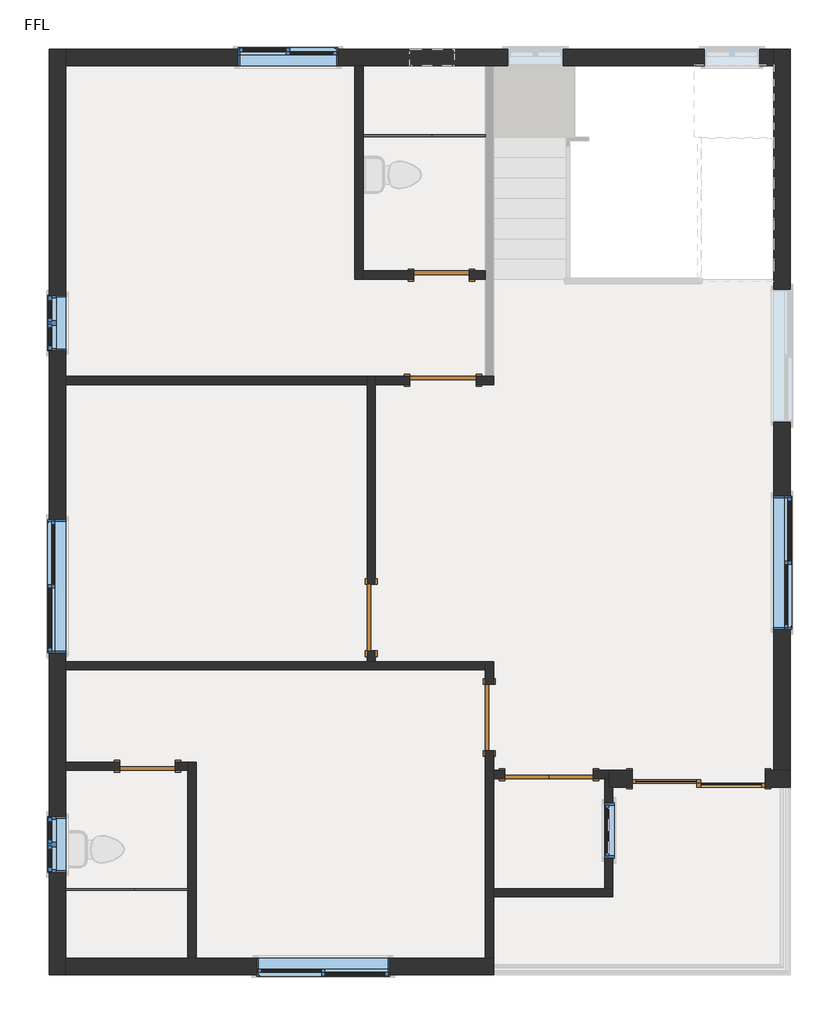
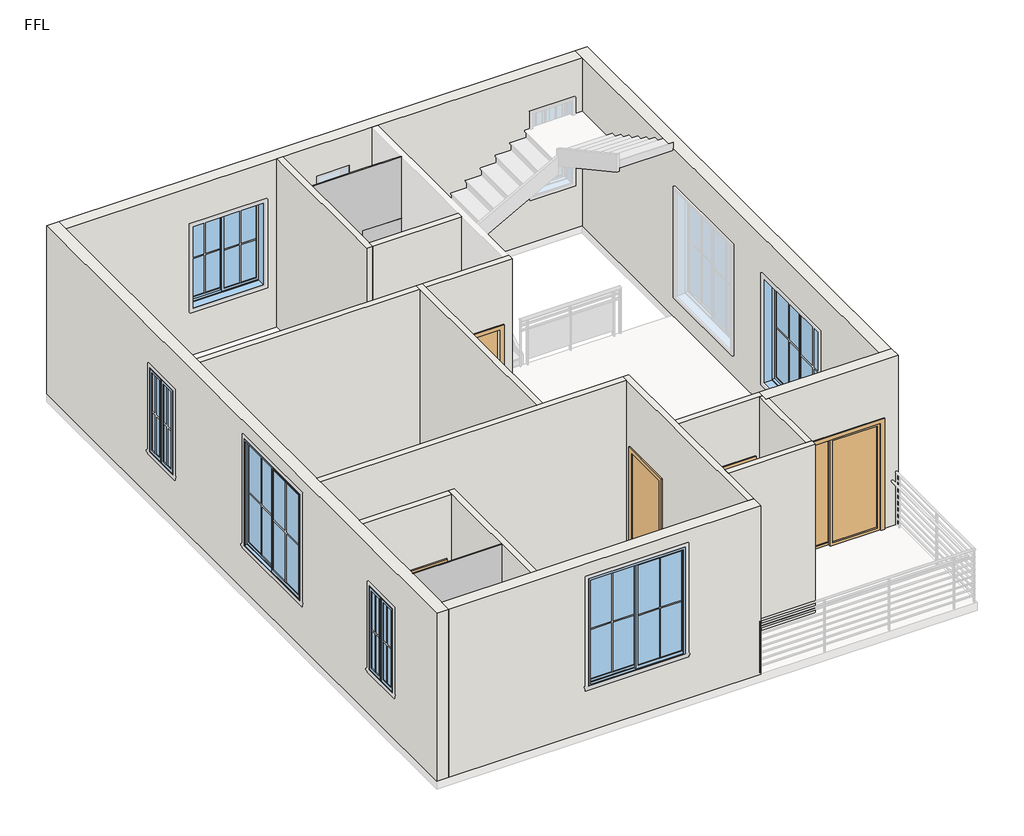
# One storey, part 1 of 3: 17 walls, 7 doors, 7 windows, 4 plates.
"""IFC4 building model written with IfcOpenShell, lengths in millimetres."""

from ifc_helpers import new_model, si_unit, frame, origin, place, context, project, spatial, polyline, outline, extrude, faceted_brep, transform, mapped, element, save
from components import door_eb8a45e1, door_d4d75d1e, door_d8f5dbb5, door_f2b275c1, door_5e62189b, door_17d80c48, system_panel_glazed_b407a8af, system_panel_glazed_ca5a80b0, window_9dcce3b5, window_5a369d27, window_5810691a, window_sliding_double_6_x7_726fea71

model = new_model("IFC4")

# Units and contexts
model_context = context("Model", 3, world=origin())
ifc_project = project(units=[si_unit("LENGTHUNIT", "METRE", prefix="MILLI")], contexts=[model_context])

# Site, building, storey
site = spatial("IfcSite", under=ifc_project)
building = spatial("IfcBuilding", under=site)
storey = spatial("IfcBuildingStorey", under=building, Name="FFL", Elevation=3505.2)

# Doors
placement = place(None, origin())
door_shape = door_eb8a45e1(model_context)
element("IfcDoor", 1, ObjectType="Door-Double-Flush_Panel : 48\" x 84\"", at=placement, inside=storey, context=model_context, shape_type="MappedRepresentation", body=[
    mapped(door_shape, transform((-7052.0133719, 2428.2295268, 3505.2), x_axis=(-1.0, 0.0, 0.0), y_axis=(0.0, -1.0, 0.0), z_axis=(0.0, 0.0, 1.0))),
])
door_2_shape = door_d4d75d1e(model_context)
element("IfcDoor", 2, ObjectType="Door-Double-Sliding : 72\" x 84\"", at=placement, inside=storey, context=model_context, shape_type="MappedRepresentation", body=[
    mapped(door_2_shape, transform((-4993.0257748, 2498.0795268, 3505.2), x_axis=(-1.0, 0.0, 0.0), y_axis=(0.0, -1.0, 0.0), z_axis=(0.0, 0.0, 1.0))),
])
door_3_shape = door_d8f5dbb5(model_context)
element("IfcDoor", 3, ObjectType="Single-Flush : 30\" x 80\"", at=placement, inside=storey, context=model_context, shape_type="MappedRepresentation", body=[
    mapped(door_3_shape, transform((-8533.1502526, 9296.8628699, 3505.2), x_axis=(1.0, 0.0, 0.0), y_axis=(0.0, 1.0, 0.0), z_axis=(0.0, 0.0, 1.0))),
])
door_4_shape = door_f2b275c1(model_context)
element("IfcDoor", 4, ObjectType="Single-Flush : 30\" x 80\"", at=placement, inside=storey, context=model_context, shape_type="MappedRepresentation", body=[
    mapped(door_4_shape, transform((-12571.8381491, 2542.5295268, 3505.2), x_axis=(1.0, 0.0, 0.0), y_axis=(0.0, 1.0, 0.0), z_axis=(0.0, 0.0, 1.0))),
])
door_5_shape = door_5e62189b(model_context)
element("IfcDoor", 5, ObjectType="Single-Flush : 36\" x 80\"", at=placement, inside=storey, context=model_context, shape_type="MappedRepresentation", body=[
    mapped(door_5_shape, transform((-9498.3502612, 4585.1627283, 3505.2), x_axis=(0.0, -1.0, 0.0), y_axis=(1.0, 0.0, 0.0), z_axis=(0.0, 0.0, 1.0))),
])
door_6_shape = door_17d80c48(model_context)
element("IfcDoor", 6, ObjectType="Single-Flush : 36\" x 80\"", at=placement, inside=storey, context=model_context, shape_type="MappedRepresentation", body=[
    mapped(door_6_shape, transform((-7872.750969, 3213.5627283, 3505.2), x_axis=(0.0, 1.0, 0.0), y_axis=(-1.0, 0.0, 0.0), z_axis=(0.0, 0.0, 1.0))),
])
element("IfcDoor", 7, ObjectType="Single-Flush : 36\" x 80\"", at=placement, inside=storey, context=model_context, shape_type="MappedRepresentation", body=[
    mapped(door_6_shape, transform((-8507.7502526, 7849.0628362, 3505.2), x_axis=(1.0, 0.0, 0.0), y_axis=(0.0, 1.0, 0.0), z_axis=(0.0, 0.0, 1.0))),
])

# Plates
system_panel_glazed_shape = system_panel_glazed_b407a8af(model_context)
element("IfcPlate", 8, ObjectType="System Panel : Glazed", at=placement, inside=storey, context=model_context, shape_type="MappedRepresentation", body=[
    mapped(system_panel_glazed_shape, transform((-12387.6881491, 816.3157145, 3505.2), x_axis=(1.0, 0.0, 0.0), y_axis=(0.0, 1.0, 0.0), z_axis=(0.0, 0.0, 1.0))),
])
element("IfcPlate", 9, ObjectType="System Panel : Glazed", at=placement, inside=storey, context=model_context, shape_type="MappedRepresentation", body=[
    mapped(system_panel_glazed_shape, transform((-8298.2002526, 11182.8127591, 3505.2), x_axis=(1.0, 0.0, 0.0), y_axis=(0.0, 1.0, 0.0), z_axis=(0.0, 0.0, 1.0))),
])
system_panel_glazed_2_shape = system_panel_glazed_ca5a80b0(model_context)
element("IfcPlate", 10, ObjectType="System Panel : Glazed", at=placement, inside=storey, context=model_context, shape_type="MappedRepresentation", body=[
    mapped(system_panel_glazed_2_shape, transform((-12857.5442008, 816.3157145, 3505.2), x_axis=(1.0, 0.0, 0.0), y_axis=(0.0, 1.0, 0.0), z_axis=(0.0, 0.0, 1.0))),
])
element("IfcPlate", 11, ObjectType="System Panel : Glazed", at=placement, inside=storey, context=model_context, shape_type="MappedRepresentation", body=[
    mapped(system_panel_glazed_2_shape, transform((-8768.1005763, 11182.8127591, 3505.2), x_axis=(1.0, 0.0, 0.0), y_axis=(0.0, 1.0, 0.0), z_axis=(0.0, 0.0, 1.0))),
])

# Walls
element("IfcWall", 12, ObjectType="10\"", at=placement, inside=storey, context=model_context, shape_type="Brep", body=[
    faceted_brep([(-13924.3002526, 12402.0128362, 3505.2), (-13924.3002526, -323.3871638, 3505.2), (-13924.3002526, -323.3871638, 6858.0), (-13924.3002526, 12402.0128362, 6858.0), (-13924.3002526, 5931.3627283, 6553.2), (-13924.3002526, 4102.5627283, 6553.2), (-13924.3002526, 4102.5627283, 4419.6), (-13924.3002526, 5931.3627283, 4419.6), (-13924.3002526, 9017.4628362, 6096.0), (-13924.3002526, 8255.4628362, 6096.0), (-13924.3002526, 8255.4628362, 4419.6), (-13924.3002526, 9017.4628362, 4419.6), (-13924.3002526, 1848.3128362, 6096.0), (-13924.3002526, 1086.3128362, 6096.0), (-13924.3002526, 1086.3128362, 4419.6), (-13924.3002526, 1848.3128362, 4419.6), (-13695.7002526, 12402.0128362, 3505.2), (-13695.7002526, 12402.0128362, 6858.0), (-13695.7002526, 12173.4128362, 6858.0), (-13695.7002526, 7906.2128362, 6858.0), (-13695.7002526, 7791.9128362, 6858.0), (-13695.7002526, 3981.9127283, 6858.0), (-13695.7002526, 3867.6127283, 6858.0), (-13695.7002526, 2599.6795268, 6858.0), (-13695.7002526, 2485.3795268, 6858.0), (-13695.7002526, -94.7871638, 6858.0), (-13695.7002526, -323.3871638, 6858.0), (-13695.7002526, -323.3871638, 3505.2), (-13695.7002526, -94.7871638, 3505.2), (-13695.7002526, 2485.3795268, 3505.2), (-13695.7002526, 2599.6795268, 3505.2), (-13695.7002526, 3867.6127283, 3505.2), (-13695.7002526, 3981.9127283, 3505.2), (-13695.7002526, 7791.9128362, 3505.2), (-13695.7002526, 7906.2128362, 3505.2), (-13695.7002526, 12173.4128362, 3505.2), (-13695.7002526, 5931.3627283, 6553.2), (-13695.7002526, 5931.3627283, 4419.6), (-13695.7002526, 4102.5627283, 4419.6), (-13695.7002526, 4102.5627283, 6553.2), (-13695.7002526, 9017.4628362, 6096.0), (-13695.7002526, 9017.4628362, 4419.6), (-13695.7002526, 8255.4628362, 4419.6), (-13695.7002526, 8255.4628362, 6096.0), (-13695.7002526, 1848.3128362, 6096.0), (-13695.7002526, 1848.3128362, 4419.6), (-13695.7002526, 1086.3128362, 4419.6), (-13695.7002526, 1086.3128362, 6096.0)], [[[0, 1, 2, 3], [4, 5, 6, 7], [8, 9, 10, 11], [12, 13, 14, 15]], [[16, 17, 18, 19, 20, 21, 22, 23, 24, 25, 26, 27, 28, 29, 30, 31, 32, 33, 34, 35], [36, 37, 38, 39], [40, 41, 42, 43], [44, 45, 46, 47]], [[1, 0, 16, 35, 34, 33, 32, 31, 30, 29, 28, 27]], [[3, 2, 26, 25, 24, 23, 22, 21, 20, 19, 18, 17]], [[2, 1, 27, 26]], [[0, 3, 17, 16]], [[37, 36, 4, 7]], [[38, 37, 7, 6]], [[39, 38, 6, 5]], [[36, 39, 5, 4]], [[41, 40, 8, 11]], [[42, 41, 11, 10]], [[43, 42, 10, 9]], [[40, 43, 9, 8]], [[45, 44, 12, 15]], [[46, 45, 15, 14]], [[47, 46, 14, 13]], [[44, 47, 13, 12]]]),
])
element("IfcWall", 13, ObjectType="10\"", at=placement, inside=storey, context=model_context, shape_type="Brep", body=[
    faceted_brep([(-13695.7002526, -323.3871638, 3505.2), (-7815.600969, -323.3871638, 3505.2), (-7815.600969, -323.3871638, 6858.0), (-13695.7002526, -323.3871638, 6858.0), (-11073.150969, -323.3871638, 6553.2), (-9244.350969, -323.3871638, 6553.2), (-9244.350969, -323.3871638, 4419.6), (-11073.150969, -323.3871638, 4419.6), (-13695.7002526, -94.7871638, 3505.2), (-13695.7002526, -94.7871638, 6858.0), (-12019.3881491, -94.7871638, 6858.0), (-11905.0881491, -94.7871638, 6858.0), (-7929.900969, -94.7871638, 6858.0), (-7815.600969, -94.7871638, 6858.0), (-7815.600969, -94.7871638, 3505.2), (-7929.900969, -94.7871638, 3505.2), (-11905.0881491, -94.7871638, 3505.2), (-12019.3881491, -94.7871638, 3505.2), (-11073.150969, -94.7871638, 6553.2), (-11073.150969, -94.7871638, 4419.6), (-9244.350969, -94.7871638, 4419.6), (-9244.350969, -94.7871638, 6553.2)], [[[0, 1, 2, 3], [4, 5, 6, 7]], [[8, 9, 10, 11, 12, 13, 14, 15, 16, 17], [18, 19, 20, 21]], [[1, 0, 8, 17, 16, 15, 14]], [[3, 2, 13, 12, 11, 10, 9]], [[0, 3, 9, 8]], [[2, 1, 14, 13]], [[19, 18, 4, 7]], [[20, 19, 7, 6]], [[21, 20, 6, 5]], [[18, 21, 5, 4]]]),
])
element("IfcWall", 14, ObjectType="10\"", at=placement, inside=storey, context=model_context, shape_type="Brep", body=[
    faceted_brep([(-6231.2757748, 2256.7795268, 3505.2), (-6174.1257748, 2256.7795268, 3505.2), (-5907.4257748, 2256.7795268, 3505.2), (-5907.4257748, 2256.7795268, 5638.8), (-4078.6257748, 2256.7795268, 5638.8), (-4078.6257748, 2256.7795268, 3505.2), (-3735.7257748, 2256.7795268, 3505.2), (-3735.7257748, 2256.7795268, 6858.0), (-6174.1257748, 2256.7795268, 6858.0), (-6231.2757748, 2256.7795268, 6858.0), (-5907.4257748, 2485.3795268, 5638.8), (-5907.4257748, 2485.3795268, 3505.2), (-6231.2757748, 2485.3795268, 3505.2), (-6231.2757748, 2485.3795268, 6858.0), (-3964.3257748, 2485.3795268, 6858.0), (-3735.7257748, 2485.3795268, 6858.0), (-3735.7257748, 2485.3795268, 3505.2), (-3964.3257748, 2485.3795268, 3505.2), (-4078.6257748, 2485.3795268, 3505.2), (-4078.6257748, 2485.3795268, 5638.8), (-6231.2757748, 2371.0795268, 3505.2), (-6231.2757748, 2371.0795268, 6858.0)], [[[0, 1, 2, 3, 4, 5, 6, 7, 8, 9]], [[10, 11, 12, 13, 14, 15, 16, 17, 18, 19]], [[12, 11, 2, 1, 0, 20]], [[18, 17, 16, 6, 5]], [[9, 8, 7, 15, 14, 13, 21]], [[0, 9, 21, 13, 12, 20]], [[7, 6, 16, 15]], [[5, 4, 19, 18]], [[3, 2, 11, 10]], [[4, 3, 10, 19]]]),
])
element("IfcWall", 15, ObjectType="10\"", at=placement, inside=storey, context=model_context, shape_type="Brep", body=[
    faceted_brep([(-3735.7257748, 2485.3795268, 3505.2), (-3735.7257748, 12402.0128362, 3505.2), (-3735.7257748, 12402.0128362, 6858.0), (-3735.7257748, 2485.3795268, 6858.0), (-3735.7257748, 4428.4795268, 6096.0), (-3735.7257748, 6257.2795268, 6096.0), (-3735.7257748, 6257.2795268, 3962.4), (-3735.7257748, 4428.4795268, 3962.4), (-3735.7257748, 7273.2795268, 6096.0), (-3735.7257748, 9102.0795268, 6096.0), (-3735.7257748, 9102.0795268, 3962.4), (-3735.7257748, 7273.2795268, 3962.4), (-3964.3257748, 2485.3795268, 3505.2), (-3964.3257748, 2485.3795268, 6858.0), (-3964.3257748, 12173.4128362, 6858.0), (-3964.3257748, 12402.0128362, 6858.0), (-3964.3257748, 12402.0128362, 3505.2), (-3964.3257748, 12173.4128362, 3505.2), (-3964.3257748, 4428.4795268, 6096.0), (-3964.3257748, 4428.4795268, 3962.4), (-3964.3257748, 6257.2795268, 3962.4), (-3964.3257748, 6257.2795268, 6096.0), (-3964.3257748, 7273.2795268, 6096.0), (-3964.3257748, 7273.2795268, 3962.4), (-3964.3257748, 9102.0795268, 3962.4), (-3964.3257748, 9102.0795268, 6096.0)], [[[0, 1, 2, 3], [4, 5, 6, 7], [8, 9, 10, 11]], [[12, 13, 14, 15, 16, 17], [18, 19, 20, 21], [22, 23, 24, 25]], [[1, 0, 12, 17, 16]], [[3, 2, 15, 14, 13]], [[0, 3, 13, 12]], [[2, 1, 16, 15]], [[19, 18, 4, 7]], [[20, 19, 7, 6]], [[21, 20, 6, 5]], [[18, 21, 5, 4]], [[23, 22, 8, 11]], [[24, 23, 11, 10]], [[25, 24, 10, 9]], [[22, 25, 9, 8]]]),
])
element("IfcWall", 16, ObjectType="10\"", at=placement, inside=storey, context=model_context, shape_type="Brep", body=[
    faceted_brep([(-7618.7502526, 12402.0128362, 5181.6), (-7618.7502526, 12402.0128362, 3505.2), (-13695.7002526, 12402.0128362, 3505.2), (-13695.7002526, 12402.0128362, 6858.0), (-3964.3257748, 12402.0128362, 6858.0), (-3964.3257748, 12402.0128362, 3505.2), (-6856.7502526, 12402.0128362, 3505.2), (-6856.7502526, 12402.0128362, 5181.6), (-9955.5502526, 12402.0128362, 6096.0), (-11327.1502526, 12402.0128362, 6096.0), (-11327.1502526, 12402.0128362, 4419.6), (-9955.5502526, 12402.0128362, 4419.6), (-8355.3502526, 12402.0128362, 6248.4), (-8964.9502526, 12402.0128362, 6248.4), (-8964.9502526, 12402.0128362, 5638.8), (-8355.3502526, 12402.0128362, 5638.8), (-4154.8257748, 12402.0128362, 6096.0), (-4916.8257748, 12402.0128362, 6096.0), (-4916.8257748, 12402.0128362, 4419.6), (-4154.8257748, 12402.0128362, 4419.6), (-13695.7002526, 12173.4128362, 3505.2), (-9720.6009, 12173.4128362, 3505.2), (-9606.3009, 12173.4128362, 3505.2), (-7929.9002526, 12173.4128362, 3505.2), (-7815.6002526, 12173.4128362, 3505.2), (-7618.7502526, 12173.4128362, 3505.2), (-7618.7502526, 12173.4128362, 5181.6), (-6856.7502526, 12173.4128362, 5181.6), (-6856.7502526, 12173.4128362, 3505.2), (-3964.3257748, 12173.4128362, 3505.2), (-3964.3257748, 12173.4128362, 6858.0), (-7815.6002526, 12173.4128362, 6858.0), (-7929.9002526, 12173.4128362, 6858.0), (-9606.3009, 12173.4128362, 6858.0), (-9720.6009, 12173.4128362, 6858.0), (-13695.7002526, 12173.4128362, 6858.0), (-9955.5502526, 12173.4128362, 6096.0), (-9955.5502526, 12173.4128362, 4419.6), (-11327.1502526, 12173.4128362, 4419.6), (-11327.1502526, 12173.4128362, 6096.0), (-8355.3502526, 12173.4128362, 6248.4), (-8355.3502526, 12173.4128362, 5638.8), (-8964.9502526, 12173.4128362, 5638.8), (-8964.9502526, 12173.4128362, 6248.4), (-4154.8257748, 12173.4128362, 6096.0), (-4154.8257748, 12173.4128362, 4419.6), (-4916.8257748, 12173.4128362, 4419.6), (-4916.8257748, 12173.4128362, 6096.0)], [[[0, 1, 2, 3, 4, 5, 6, 7], [8, 9, 10, 11], [12, 13, 14, 15], [16, 17, 18, 19]], [[20, 21, 22, 23, 24, 25, 26, 27, 28, 29, 30, 31, 32, 33, 34, 35], [36, 37, 38, 39], [40, 41, 42, 43], [44, 45, 46, 47]], [[6, 5, 29, 28]], [[2, 1, 25, 24, 23, 22, 21, 20]], [[4, 3, 35, 34, 33, 32, 31, 30]], [[5, 4, 30, 29]], [[3, 2, 20, 35]], [[37, 36, 8, 11]], [[38, 37, 11, 10]], [[39, 38, 10, 9]], [[36, 39, 9, 8]], [[41, 40, 12, 15]], [[42, 41, 15, 14]], [[43, 42, 14, 13]], [[40, 43, 13, 12]], [[28, 27, 7, 6]], [[26, 25, 1, 0]], [[27, 26, 0, 7]], [[45, 44, 16, 19]], [[46, 45, 19, 18]], [[47, 46, 18, 17]], [[44, 47, 17, 16]]]),
])
element("IfcWall", 17, ObjectType="5\"", at=placement, inside=storey, context=model_context, shape_type="Brep", body=[
    faceted_brep([(-7815.600969, 3670.7627283, 5537.2), (-7815.600969, 3670.7627283, 3505.2), (-7815.600969, 3981.9127283, 3505.2), (-7815.600969, 3981.9127283, 6858.0), (-7815.600969, 2485.3795268, 6858.0), (-7815.600969, 2371.0795268, 6858.0), (-7815.600969, 859.7795149, 6858.0), (-7815.600969, 745.4795149, 6858.0), (-7815.600969, -94.7871638, 6858.0), (-7815.600969, -94.7871638, 3505.2), (-7815.600969, 745.4795149, 3505.2), (-7815.600969, 859.7795149, 3505.2), (-7815.600969, 2371.0795268, 3505.2), (-7815.600969, 2485.3795268, 3505.2), (-7815.600969, 2756.3627283, 3505.2), (-7815.600969, 2756.3627283, 5537.2), (-7929.900969, 3981.9127283, 3505.2), (-7929.900969, 3867.6127283, 3505.2), (-7929.900969, 3670.7627283, 3505.2), (-7929.900969, 3670.7627283, 5537.2), (-7929.900969, 2756.3627283, 5537.2), (-7929.900969, 2756.3627283, 3505.2), (-7929.900969, -94.7871638, 3505.2), (-7929.900969, -94.7871638, 6858.0), (-7929.900969, 3867.6127283, 6858.0), (-7929.900969, 3981.9127283, 6858.0)], [[[0, 1, 2, 3, 4, 5, 6, 7, 8, 9, 10, 11, 12, 13, 14, 15]], [[16, 17, 18, 19, 20, 21, 22, 23, 24, 25]], [[2, 1, 18, 17, 16]], [[14, 13, 12, 11, 10, 9, 22, 21]], [[8, 7, 6, 5, 4, 3, 25, 24, 23]], [[9, 8, 23, 22]], [[3, 2, 16, 25]], [[19, 18, 1, 0]], [[20, 19, 0, 15]], [[21, 20, 15, 14]]]),
])
element("IfcWall", 18, ObjectType="5\"", at=placement, inside=storey, context=model_context, shape_type="Brep", body=[
    faceted_brep([(-7929.900969, 3981.9127283, 3505.2), (-9441.2002612, 3981.9127283, 3505.2), (-9555.5002612, 3981.9127283, 3505.2), (-13695.7002526, 3981.9127283, 3505.2), (-13695.7002526, 3981.9127283, 6858.0), (-9555.5002612, 3981.9127283, 6858.0), (-9441.2002612, 3981.9127283, 6858.0), (-7929.900969, 3981.9127283, 6858.0), (-7929.900969, 3867.6127283, 3505.2), (-7929.900969, 3867.6127283, 6858.0), (-13695.7002526, 3867.6127283, 6858.0), (-13695.7002526, 3867.6127283, 3505.2)], [[[0, 1, 2, 3, 4, 5, 6, 7]], [[8, 9, 10, 11]], [[3, 2, 1, 0, 8, 11]], [[7, 6, 5, 4, 10, 9]], [[0, 7, 9, 8]], [[4, 3, 11, 10]]]),
])
element("IfcWall", 19, ObjectType="5\"", at=placement, inside=storey, context=model_context, shape_type="Brep", body=[
    faceted_brep([(-9441.2002612, 3981.9127283, 3505.2), (-9441.2002612, 4127.9627283, 3505.2), (-9441.2002612, 4127.9627283, 5537.2), (-9441.2002612, 5042.3627283, 5537.2), (-9441.2002612, 5042.3627283, 3505.2), (-9441.2002612, 7791.9128362, 3505.2), (-9441.2002612, 7906.2128362, 3505.2), (-9441.2002612, 7906.2128362, 6858.0), (-9441.2002612, 7791.9128362, 6858.0), (-9441.2002612, 3981.9127283, 6858.0), (-9555.5002612, 4127.9627283, 5537.2), (-9555.5002612, 4127.9627283, 3505.2), (-9555.5002612, 3981.9127283, 3505.2), (-9555.5002612, 3981.9127283, 6858.0), (-9555.5002612, 7791.9128362, 6858.0), (-9555.5002612, 7906.2128362, 6858.0), (-9555.5002612, 7906.2128362, 3505.2), (-9555.5002612, 7791.9128362, 3505.2), (-9555.5002612, 5042.3627283, 3505.2), (-9555.5002612, 5042.3627283, 5537.2)], [[[0, 1, 2, 3, 4, 5, 6, 7, 8, 9]], [[10, 11, 12, 13, 14, 15, 16, 17, 18, 19]], [[12, 11, 1, 0]], [[18, 17, 16, 6, 5, 4]], [[9, 8, 7, 15, 14, 13]], [[0, 9, 13, 12]], [[7, 6, 16, 15]], [[2, 1, 11, 10]], [[3, 2, 10, 19]], [[4, 3, 19, 18]]]),
])
element("IfcWall", 20, ObjectType="5\"", at=placement, inside=storey, context=model_context, shape_type="SweptSolid", body=[
    extrude(outline(polyline([(-13695.7002526, 7906.2128362), (-9555.5002612, 7906.2128362), (-9555.5002612, 7791.9128362), (-13695.7002526, 7791.9128362), (-13695.7002526, 7906.2128362)])), frame((0.0, 0.0, 3505.2), z_axis=(0.0, 0.0, 1.0), x_axis=(1.0, 0.0, 0.0)), (0.0, 0.0, 1.0), 3352.8),
])
element("IfcWall", 21, ObjectType="5\"", at=placement, inside=storey, context=model_context, shape_type="Brep", body=[
    faceted_brep([(-8050.5502526, 7791.9128362, 5537.2), (-8050.5502526, 7791.9128362, 3505.2), (-7815.6002526, 7791.9128362, 3505.2), (-7815.6002526, 7791.9128362, 6858.0), (-9441.2002612, 7791.9128362, 6858.0), (-9441.2002612, 7791.9128362, 3505.2), (-8964.9502526, 7791.9128362, 3505.2), (-8964.9502526, 7791.9128362, 5537.2), (-7815.6002526, 7906.2128362, 3505.2), (-7929.9002526, 7906.2128362, 3505.2), (-8050.5502526, 7906.2128362, 3505.2), (-8050.5502526, 7906.2128362, 5537.2), (-8964.9502526, 7906.2128362, 5537.2), (-8964.9502526, 7906.2128362, 3505.2), (-9441.2002612, 7906.2128362, 3505.2), (-9441.2002612, 7906.2128362, 6858.0), (-7929.9002526, 7906.2128362, 6858.0), (-7815.6002526, 7906.2128362, 6858.0)], [[[0, 1, 2, 3, 4, 5, 6, 7]], [[8, 9, 10, 11, 12, 13, 14, 15, 16, 17]], [[6, 5, 14, 13]], [[2, 1, 10, 9, 8]], [[4, 3, 17, 16, 15]], [[5, 4, 15, 14]], [[3, 2, 8, 17]], [[11, 10, 1, 0]], [[12, 11, 0, 7]], [[13, 12, 7, 6]]]),
])
element("IfcWall", 22, ObjectType="5\"", at=placement, inside=storey, context=model_context, shape_type="Brep", body=[
    faceted_brep([(-9720.6009, 12173.4128362, 3505.2), (-9720.6009, 9239.7128699, 3505.2), (-9720.6009, 9239.7128699, 6858.0), (-9720.6009, 12173.4128362, 6858.0), (-9606.3009, 12173.4128362, 3505.2), (-9606.3009, 12173.4128362, 6858.0), (-9606.3009, 9354.0128699, 6858.0), (-9606.3009, 9239.7128699, 6858.0), (-9606.3009, 9239.7128699, 3505.2), (-9606.3009, 9354.0128699, 3505.2)], [[[0, 1, 2, 3]], [[4, 5, 6, 7, 8, 9]], [[1, 0, 4, 9, 8]], [[3, 2, 7, 6, 5]], [[0, 3, 5, 4]], [[2, 1, 8, 7]]]),
])
element("IfcWall", 23, ObjectType="5\"", at=placement, inside=storey, context=model_context, shape_type="SweptSolid", body=[
    extrude(outline(polyline([(5537.2, -8152.1502526), (3505.2, -8152.1502526), (3505.2, -7929.9002526), (6858.0, -7929.9002526), (6858.0, -9606.3009), (3505.2, -9606.3009), (3505.2, -8914.1502526), (5537.2, -8914.1502526), (5537.2, -8152.1502526)])), frame((0.0, 9239.7128699, 0.0), z_axis=(0.0, 1.0, 0.0), x_axis=(0.0, 0.0, 1.0)), (0.0, 0.0, 1.0), 114.3),
])
element("IfcWall", 24, ObjectType="5\"", at=placement, inside=storey, context=model_context, shape_type="Brep", body=[
    faceted_brep([(-7815.600969, 2485.3795268, 6858.0), (-6231.2757748, 2485.3795268, 6858.0), (-6231.2757748, 2485.3795268, 3505.2), (-6442.4133719, 2485.3795268, 3505.2), (-6442.4133719, 2485.3795268, 5638.8), (-7661.6133719, 2485.3795268, 5638.8), (-7661.6133719, 2485.3795268, 3505.2), (-7815.600969, 2485.3795268, 3505.2), (-6231.2757748, 2371.0795268, 6858.0), (-6288.4257748, 2371.0795268, 6858.0), (-7815.600969, 2371.0795268, 6858.0), (-7815.600969, 2371.0795268, 3505.2), (-7661.6133719, 2371.0795268, 3505.2), (-7661.6133719, 2371.0795268, 5638.8), (-6442.4133719, 2371.0795268, 5638.8), (-6442.4133719, 2371.0795268, 3505.2), (-6288.4257748, 2371.0795268, 3505.2), (-6231.2757748, 2371.0795268, 3505.2)], [[[0, 1, 2, 3, 4, 5, 6, 7]], [[8, 9, 10, 11, 12, 13, 14, 15, 16, 17]], [[2, 17, 16, 15, 3]], [[11, 7, 6, 12]], [[1, 0, 10, 9, 8]], [[2, 1, 8, 17]], [[0, 7, 11, 10]], [[5, 13, 12, 6]], [[13, 5, 4, 14]], [[14, 4, 3, 15]]]),
])
element("IfcWall", 25, ObjectType="5\"", at=placement, inside=storey, context=model_context, shape_type="Brep", body=[
    faceted_brep([(-7815.600969, 745.4795149, 3505.2), (-6174.1257748, 745.4795149, 3505.2), (-6174.1257748, 745.4795149, 6858.0), (-7815.600969, 745.4795149, 6858.0), (-7815.600969, 859.7795149, 3505.2), (-7815.600969, 859.7795149, 6858.0), (-6288.4257748, 859.7795149, 6858.0), (-6174.1257748, 859.7795149, 6858.0), (-6174.1257748, 859.7795149, 3505.2), (-6288.4257748, 859.7795149, 3505.2)], [[[0, 1, 2, 3]], [[4, 5, 6, 7, 8, 9]], [[1, 0, 4, 9, 8]], [[3, 2, 7, 6, 5]], [[0, 3, 5, 4]], [[2, 1, 8, 7]]]),
])
element("IfcWall", 26, ObjectType="5\"", at=placement, inside=storey, context=model_context, shape_type="Brep", body=[
    faceted_brep([(-6174.1257748, 859.7795149, 3505.2), (-6174.1257748, 2256.7795268, 3505.2), (-6174.1257748, 2256.7795268, 6858.0), (-6174.1257748, 859.7795149, 6858.0), (-6174.1257748, 2040.8795268, 5588.0), (-6174.1257748, 2040.8795268, 4419.6), (-6174.1257748, 1278.8795268, 4419.6), (-6174.1257748, 1278.8795268, 5588.0), (-6288.4257748, 859.7795149, 3505.2), (-6288.4257748, 859.7795149, 6858.0), (-6288.4257748, 2371.0795268, 6858.0), (-6288.4257748, 2371.0795268, 3505.2), (-6288.4257748, 2040.8795268, 5588.0), (-6288.4257748, 1278.8795268, 5588.0), (-6288.4257748, 1278.8795268, 4419.6), (-6288.4257748, 2040.8795268, 4419.6), (-6231.2757748, 2371.0795268, 3505.2), (-6231.2757748, 2256.7795268, 3505.2), (-6231.2757748, 2256.7795268, 6858.0), (-6231.2757748, 2371.0795268, 6858.0)], [[[0, 1, 2, 3], [4, 5, 6, 7]], [[8, 9, 10, 11], [12, 13, 14, 15]], [[1, 0, 8, 11, 16, 17]], [[3, 2, 18, 19, 10, 9]], [[0, 3, 9, 8]], [[2, 1, 17, 18]], [[17, 16, 19, 18]], [[16, 11, 10, 19]], [[5, 4, 12, 15]], [[6, 5, 15, 14]], [[7, 6, 14, 13]], [[4, 7, 13, 12]]]),
])
element("IfcWall", 27, ObjectType="5\"", at=placement, inside=storey, context=model_context, shape_type="Brep", body=[
    faceted_brep([(-11905.0881491, -94.7871638, 3505.2), (-11905.0881491, 2599.6795268, 3505.2), (-11905.0881491, 2599.6795268, 6858.0), (-11905.0881491, -94.7871638, 6858.0), (-12019.3881491, -94.7871638, 3505.2), (-12019.3881491, -94.7871638, 6858.0), (-12019.3881491, 2485.3795268, 6858.0), (-12019.3881491, 2599.6795268, 6858.0), (-12019.3881491, 2599.6795268, 3505.2), (-12019.3881491, 2485.3795268, 3505.2)], [[[0, 1, 2, 3]], [[4, 5, 6, 7, 8, 9]], [[1, 0, 4, 9, 8]], [[3, 2, 7, 6, 5]], [[0, 3, 5, 4]], [[2, 1, 8, 7]]]),
])
element("IfcWall", 28, ObjectType="5\"", at=placement, inside=storey, context=model_context, shape_type="SweptSolid", body=[
    extrude(outline(polyline([(5537.2, -12190.8381491), (3505.2, -12190.8381491), (3505.2, -12019.3881491), (6858.0, -12019.3881491), (6858.0, -13695.7002526), (3505.2, -13695.7002526), (3505.2, -12952.8381491), (5537.2, -12952.8381491), (5537.2, -12190.8381491)])), frame((0.0, 2485.3795268, 0.0), z_axis=(0.0, 1.0, 0.0), x_axis=(0.0, 0.0, 1.0)), (0.0, 0.0, 1.0), 114.3),
])

# Windows
window_shape = window_9dcce3b5(model_context)
element("IfcWindow", 29, ObjectType="Window-Casement-Double : 2'-6\" X 5'-6\"", at=placement, inside=storey, context=model_context, shape_type="MappedRepresentation", body=[
    mapped(window_shape, transform((-13810.0002526, 8636.4628362, 3505.2), x_axis=(0.0, 1.0, 0.0), y_axis=(-1.0, 0.0, 0.0), z_axis=(0.0, 0.0, 1.0))),
])
element("IfcWindow", 30, ObjectType="Window-Casement-Double : 2'-6\" X 5'-6\"", at=placement, inside=storey, context=model_context, shape_type="MappedRepresentation", body=[
    mapped(window_shape, transform((-13810.0002526, 1467.3128362, 3505.2), x_axis=(0.0, 1.0, 0.0), y_axis=(-1.0, 0.0, 0.0), z_axis=(0.0, 0.0, 1.0))),
])
window_2_shape = window_5a369d27(model_context)
element("IfcWindow", 31, ObjectType="Window-Double-Hung : 30\" x 46\"", at=placement, inside=storey, context=model_context, shape_type="MappedRepresentation", body=[
    mapped(window_2_shape, transform((-6231.2757748, 1659.8795268, 3505.2), x_axis=(0.0, -1.0, 0.0), y_axis=(1.0, 0.0, 0.0), z_axis=(0.0, 0.0, 1.0))),
])
window_3_shape = window_5810691a(model_context)
element("IfcWindow", 32, ObjectType="Window-Sliding-Double : 54\" x 66\"", at=placement, inside=storey, context=model_context, shape_type="MappedRepresentation", body=[
    mapped(window_3_shape, transform((-10641.3502526, 12291.5228362, 3505.2), x_axis=(1.0, 0.0, 0.0), y_axis=(0.0, 1.0, 0.0), z_axis=(0.0, 0.0, 1.0))),
])
window_sliding_double_6_x7_shape = window_sliding_double_6_x7_726fea71(model_context)
element("IfcWindow", 33, ObjectType="Window-Sliding-Double : 6'X7'", at=placement, inside=storey, context=model_context, shape_type="MappedRepresentation", body=[
    mapped(window_sliding_double_6_x7_shape, transform((-10158.750969, -212.8971638, 3505.2), x_axis=(-1.0, 0.0, 0.0), y_axis=(0.0, -1.0, 0.0), z_axis=(0.0, 0.0, 1.0))),
])
element("IfcWindow", 34, ObjectType="Window-Sliding-Double : 6'X7'", at=placement, inside=storey, context=model_context, shape_type="MappedRepresentation", body=[
    mapped(window_sliding_double_6_x7_shape, transform((-13813.8102526, 5016.9627283, 3505.2), x_axis=(0.0, 1.0, 0.0), y_axis=(-1.0, 0.0, 0.0), z_axis=(0.0, 0.0, 1.0))),
])
element("IfcWindow", 35, ObjectType="Window-Sliding-Double : 6'X7'", at=placement, inside=storey, context=model_context, shape_type="MappedRepresentation", body=[
    mapped(window_sliding_double_6_x7_shape, transform((-3846.2157748, 5342.8795268, 3048.0), x_axis=(0.0, -1.0, 0.0), y_axis=(1.0, 0.0, 0.0), z_axis=(0.0, 0.0, 1.0))),
])

save(model, "model.ifc")

# Revit data of these elements
# Type "Door-Double-Flush_Panel : 48\" x 84\""
#   Type Mark = "11"
#   Construction Type Id = "DOOR"
#   Assembly Code = "C1020"
#   Analytic Construction = "Wooden"
#   Thickness = 0' - 2"
#   Thermal Resistance (R) = 2.5876 (h·ft²·°F)/BTU
#   Swing Angle [instance default] = 90.00°
#   Panel Width = 2' - 0"
#   Heat Transfer Coefficient (U) = 0.3865 BTU/(h·ft²·°F)
#   Height = 7' - 0"
#   Trim Projection Ext = 0' - 1"
#   Trim Projection Int = 0' - 1"
#   Trim Width = 0' - 3"
#   Width = 4' - 0"
#   Define Thermal Properties by = 1
#   Panel Material = Wood - Birch - Solid Stained Light Low Gloss
#   Trim Material = Paint - Sienna
#   Visual Light Transmittance = 0
#   Solar Heat Gain Coefficient = 0
#   Function = (empty or 0)
#   Wall Closure = (empty or 0)
# Type "Door-Double-Sliding : 72\" x 84\""
#   Type Mark = "10"
#   Construction Type Id = "opn-d45"
#   Assembly Code = "C1020"
#   Analytic Construction = "Wood frame, double glass door "
#   Thickness = 0' - 2"
#   Thermal Resistance (R) = 1.8150 (h·ft²·°F)/BTU
#   Heat Transfer Coefficient (U) = 0.5510 BTU/(h·ft²·°F)
#   Height = 7' - 0"
#   Rail Width = 0' - 2"
#   Stiles = 0' - 2"
#   Trim Projection Ext = 0' - 1"
#   Trim Projection Int = 0' - 1"
#   Trim Width = 0' - 3"
#   Width = 6' - 0"
#   Define Thermal Properties by = 1
#   Glazing = Glass
#   Panel Material = Wood - Birch - Solid Stained Light Low Gloss
#   Trim Material = Paint - Sienna
#   Visual Light Transmittance = 0
#   Solar Heat Gain Coefficient = 0
#   Function = (empty or 0)
#   Wall Closure = (empty or 0)
# Type "Single-Flush : 30\" x 80\""
#   Type Mark = "5"
#   Construction Type Id = "MDOOR"
#   Assembly Code = "C1020"
#   Analytic Construction = "Metal"
#   Thickness = 0' - 2"
#   Heat Transfer Coefficient (U) = 0.651978 BTU/(h·ft²·°F)
#   Height = 6' - 8"
#   Trim Projection Ext = 0' - 1"
#   Trim Projection Int = 0' - 1"
#   Trim Width = 0' - 3"
#   Width = 2' - 6"
#   Define Thermal Properties by = 1
#   Define Thermal Properties by = 1
#   Door Material = Door - Panel
#   Frame Material = Door - Frame
#   Visual Light Transmittance = 0
#   Solar Heat Gain Coefficient = 0
#   Function = (empty or 0)
#   Wall Closure = (empty or 0)
# Type "Single-Flush : 36\" x 80\""
#   Type Mark = "6"
#   Construction Type Id = "MDOOR"
#   Assembly Code = "C1020"
#   Analytic Construction = "Metal"
#   Thickness = 0' - 2"
#   Heat Transfer Coefficient (U) = 0.651978 BTU/(h·ft²·°F)
#   Height = 6' - 8"
#   Trim Projection Ext = 0' - 1"
#   Trim Projection Int = 0' - 1"
#   Trim Width = 0' - 3"
#   Width = 3' - 0"
#   Define Thermal Properties by = 1
#   Define Thermal Properties by = 1
#   Door Material = Door - Panel
#   Frame Material = Door - Frame
#   Visual Light Transmittance = 0
#   Solar Heat Gain Coefficient = 0
#   Function = (empty or 0)
#   Wall Closure = (empty or 0)
# Type "System Panel : Glazed"
#   Construction Type Id = "GSP4R"
#   Analytic Construction = "1/8 in Pilkington single glazing"
#   Visual Light Transmittance = 0.9
#   Solar Heat Gain Coefficient = 0.86
#   Heat Transfer Coefficient (U) = 1.18115 BTU/(h·ft²·°F)
#   Define Thermal Properties by = 1
# Type "10\""
#   Assembly Code = "B2010"
#   Layers, outside or top first: 0' - 9" "Gypsum Wall Board" (function 1)
# Type "5\""
#   Assembly Code = "B2010"
#   Layers, outside or top first: 0' - 4 1/2" "Gypsum Wall Board" (function 1)
# Type "Window-Casement-Double : 2'-6\" X 5'-6\""
#   Type Mark = "21"
#   Fire Rating = "0.5h"
#   Assembly Code = "B2020100"
#   Analytic Construction = "Double glazing - domestic"
#   Frame Extension [instance default] = 0' - 0 1/4"
#   Window Inset [instance default] = 0' - 0"
#   Wall Thickness [instance default] = 0' - 6"
#   Interior Wall Closure [instance default] = 0' - 2 1/4"
#   Half Width = 1' - 3"
#   Visual Light Transmittance = 0.81
#   Thermal Resistance (R) = 1.8146 (h·ft²·°F)/BTU
#   Solar Heat Gain Coefficient = 0.76
#   Rough Width = 2' - 6 1/2"
#   Rough Height = 5' - 6 1/2"
#   Height = 5' - 6"
#   Heat Transfer Coefficient (U) = 0.5511 BTU/(h·ft²·°F)
#   Exterior Wall Closure [instance default] = 0' - 1 1/4"
#   Extension Jamb [instance default] = 0' - 2 1/4"
#   Default Sill Height = 3' - 0"
#   Width = 2' - 6"
#   Muntin Visibility = yes
#   Interior Trim Visibility [instance default] = yes
#   Exterior Trim Visibility [instance default] = yes
#   Extension Jamb Visibility [instance default] = yes
#   Interior Trim Material = Wood - Stained
#   Muntin Pattern = Muntin Pattern_2x2 : Muntin Pattern_2x2
#   Interior Trim = Trim-Window-Interior-Flat : Picture Frame
#   Interior Frame Material = Wood - Stained
#   Glass Panel Material = Glass
#   Exterior Trim Material = Clad - White
#   Exterior Trim = Trim-Window-Exterior-Flat : with Sill
#   Exterior Frame Material = Clad - White
#   Wall Closure = (empty or 0)
# Type "Window-Double-Hung : 30\" x 46\""
#   Type Mark = "13"
#   Fire Rating = "0.5h"
#   Construction Type Id = "DG-DR"
#   Assembly Code = "B2020100"
#   Analytic Construction = "Double glazing - domestic"
#   Wall Thickness [instance default] = 0' - 6"
#   Window Inset [instance default] = 0' - 0"
#   Visual Light Transmittance = 0.81
#   Thermal Resistance (R) = 1.8146 (h·ft²·°F)/BTU
#   Solar Heat Gain Coefficient = 0.76
#   Muntin Width = 2' - 0"
#   Muntin Height = 1' - 7 1/8"
#   Interior Wall Closure [instance default] = 0' - 1 1/2"
#   Rough Width = 2' - 6 1/2"
#   Rough Height = 3' - 10 1/2"
#   Frame Extension [instance default] = 0' - 1 1/4"
#   Exterior Wall Closure [instance default] = 0' - 0 1/2"
#   Extension Jamb [instance default] = 0' - 1 1/2"
#   Heat Transfer Coefficient (U) = 0.5511 BTU/(h·ft²·°F)
#   Height = 3' - 10"
#   Width = 2' - 6"
#   Define Thermal Properties by = 1
#   Top Muntin Visibility = yes
#   Indicator Visibility [instance default] = yes
#   Extension Jamb Visibility [instance default] = yes
#   Interior Trim Visibility [instance default] = yes
#   Exterior Trim Visibility [instance default] = yes
#   Define Thermal Properties by = 1
#   Bottom Muntin Visibility = yes
#   Muntin Pattern = Muntin Pattern_2x2 : Muntin Pattern_2x2
#   Interior Trim Material = Wood - Stained
#   Interior Trim = Trim-Window-Interior-Flat : Picture Frame
#   Exterior Trim Material = Clad - White
#   Exterior Trim = Trim-Window-Exterior-Flat : with Sill
#   Glass Panel Material = Glass
#   Exterior Frame Material = Clad - White
#   Interior Frame Material = Wood - Stained
#   Wall Closure = (empty or 0)
# Type "Window-Sliding-Double : 54\" x 66\""
#   Type Mark = "20"
#   Fire Rating = "0.5h"
#   Assembly Code = "B2020100"
#   Analytic Construction = "Double glazing - domestic"
#   Window Inset [instance default] = 0' - 0"
#   Wall Thickness [instance default] = 0' - 6"
#   Visual Light Transmittance = 0.81
#   Thermal Resistance (R) = 1.8146 (h·ft²·°F)/BTU
#   Solar Heat Gain Coefficient = 0.76
#   Muntin Width = 1' - 11 5/8"
#   Muntin Height = 5' - 0 1/4"
#   Interior Wall Closure [instance default] = 0' - 2 3/4"
#   Heat Transfer Coefficient (U) = 0.5511 BTU/(h·ft²·°F)
#   Frame Extension [instance default] = 0' - 0 1/4"
#   Exterior Wall Closure [instance default] = 0' - 1 1/4"
#   Rough Width = 4' - 6 1/2"
#   Rough Height = 5' - 6 1/2"
#   Height = 5' - 6"
#   Extension Jamb [instance default] = 0' - 2 3/4"
#   Default Sill Height = 3' - 0"
#   Width = 4' - 6"
#   Interior Trim Visibility [instance default] = yes
#   Indicator Visibility [instance default] = yes
#   Exterior Trim Visibility [instance default] = yes
#   Muntin Visibility = yes
#   Extension Jamb Visibility [instance default] = yes
#   Muntin Pattern = Muntin Pattern_2x2 : Muntin Pattern_2x2
#   Interior Trim Material = Wood - Stained
#   Interior Trim = Trim-Window-Interior-Flat : Picture Frame
#   Interior Frame Material = Wood - Stained
#   Glass Panel Material = Glass
#   Exterior Trim Material = Clad - White
#   Exterior Trim = Trim-Window-Exterior-Flat : with Sill
#   Exterior Frame Material = Clad - White
#   Wall Closure = (empty or 0)
# Type "Window-Sliding-Double : 6'X7'"
#   Type Mark = "19"
#   Fire Rating = "0.5h"
#   Assembly Code = "B2020100"
#   Analytic Construction = "Double glazing - domestic"
#   Window Inset [instance default] = 0' - 0"
#   Wall Thickness [instance default] = 0' - 6"
#   Visual Light Transmittance = 0.81
#   Thermal Resistance (R) = 1.8146 (h·ft²·°F)/BTU
#   Solar Heat Gain Coefficient = 0.76
#   Muntin Width = 2' - 8 5/8"
#   Muntin Height = 6' - 6 1/4"
#   Interior Wall Closure [instance default] = 0' - 2 3/4"
#   Heat Transfer Coefficient (U) = 0.5511 BTU/(h·ft²·°F)
#   Frame Extension [instance default] = 0' - 0 1/4"
#   Exterior Wall Closure [instance default] = 0' - 1 1/4"
#   Rough Width = 6' - 0 1/2"
#   Rough Height = 7' - 0 1/2"
#   Height = 7' - 0"
#   Extension Jamb [instance default] = 0' - 2 3/4"
#   Default Sill Height = 3' - 0"
#   Width = 6' - 0"
#   Interior Trim Visibility [instance default] = yes
#   Indicator Visibility [instance default] = yes
#   Exterior Trim Visibility [instance default] = yes
#   Muntin Visibility = yes
#   Extension Jamb Visibility [instance default] = yes
#   Muntin Pattern = Muntin Pattern_2x2 : Muntin Pattern_2x2
#   Interior Trim Material = Wood - Stained
#   Interior Trim = Trim-Window-Interior-Flat : Picture Frame
#   Interior Frame Material = Wood - Stained
#   Glass Panel Material = Glass
#   Exterior Trim Material = Clad - White
#   Exterior Trim = Trim-Window-Exterior-Flat : with Sill
#   Exterior Frame Material = Clad - White
#   Wall Closure = (empty or 0)
# Element 1 (IfcDoor, "Door-Double-Flush_Panel : 48\" x 84\"")
#   Swing Angle = 90.00°
#   Phase Created = New Construction
#   Materials on its faces: "Paint - Sienna", "Wood - Birch - Solid Stained Light Low Gloss"
# Element 2 (IfcDoor, "Door-Double-Sliding : 72\" x 84\"")
#   Phase Created = New Construction
#   Materials on its faces: "Paint - Sienna", "Wood - Birch - Solid Stained Light Low Gloss", "Glass"
# Elements 3, 4 (IfcDoor, "Single-Flush : 30\" x 80\"")
#   Phase Created = New Construction
#   Materials on its faces: "Door - Frame", "Door - Panel"
# Elements 5, 6, 7 (IfcDoor, "Single-Flush : 36\" x 80\"")
#   Phase Created = New Construction
#   Materials on its faces: "Door - Frame", "Door - Panel"
# Elements 8, 9, 10, 11 (IfcPlate, "System Panel : Glazed")
#   Phase Created = New Construction
#   Materials on its faces: "Glass"
# Elements 12, 13, 14, 15, 16 (IfcWall, "10\"")
#   Top Offset = 0' - 0"
#   Base Offset = 0' - 0"
#   Unconnected Height = 11' - 0"
#   wall height = 11' - 0"
#   Phase Created = New Construction
#   Base Constraint = FFL
#   Materials on its faces: "Gypsum Wall Board"
# Elements 17, 18, 19, 20, 21, 22, 23, 24, 25, 26, 27, 28 (IfcWall, "5\"")
#   Top Offset = 0' - 0"
#   Base Offset = 0' - 0"
#   Unconnected Height = 11' - 0"
#   wall height = 11' - 0"
#   Phase Created = New Construction
#   Base Constraint = FFL
#   Materials on its faces: "Gypsum Wall Board"
# Element 29 (IfcWindow, "Window-Casement-Double : 2'-6\" X 5'-6\"")
#   Mark = "17"
#   Window Inset = 0' - 0"
#   Interior Wall Closure = 0' - 2 1/4"
#   Frame Extension = 0' - 0 1/4"
#   Exterior Wall Closure = 0' - 1 1/4"
#   Interior Trim Visibility = yes
#   Exterior Trim Visibility = yes
#   Phase Created = New Construction
#   Materials on its faces: "Wood - Stained", "Glass", "Clad - White"
# Element 30 (IfcWindow, "Window-Casement-Double : 2'-6\" X 5'-6\"")
#   Mark = "18"
#   Window Inset = 0' - 0"
#   Interior Wall Closure = 0' - 2 1/4"
#   Frame Extension = 0' - 0 1/4"
#   Exterior Wall Closure = 0' - 1 1/4"
#   Interior Trim Visibility = yes
#   Exterior Trim Visibility = yes
#   Phase Created = New Construction
#   Materials on its faces: "Wood - Stained", "Glass", "Clad - White"
# Element 31 (IfcWindow, "Window-Double-Hung : 30\" x 46\"")
#   Mark = "11"
#   Window Inset = 0' - 0"
#   Interior Wall Closure = 0' - 1 1/2"
#   Frame Extension = 0' - 1 1/4"
#   Exterior Wall Closure = 0' - 0 1/2"
#   Interior Trim Visibility = yes
#   Indicator Visibility = yes
#   Exterior Trim Visibility = yes
#   Phase Created = New Construction
#   Materials on its faces: "Wood - Stained", "Glass", "Clad - White"
# Element 32 (IfcWindow, "Window-Sliding-Double : 54\" x 66\"")
#   Mark = "16"
#   Window Inset = 0' - 0"
#   Interior Wall Closure = 0' - 2 3/4"
#   Frame Extension = 0' - 0 1/4"
#   Exterior Wall Closure = 0' - 1 1/4"
#   Interior Trim Visibility = yes
#   Indicator Visibility = yes
#   Exterior Trim Visibility = yes
#   Phase Created = New Construction
#   Materials on its faces: "Wood - Stained", "Glass", "Clad - White"
# Element 33 (IfcWindow, "Window-Sliding-Double : 6'X7'")
#   Mark = "12"
#   Window Inset = 0' - 0"
#   Interior Wall Closure = 0' - 2 3/4"
#   Frame Extension = 0' - 0 1/4"
#   Exterior Wall Closure = 0' - 1 1/4"
#   Interior Trim Visibility = yes
#   Indicator Visibility = yes
#   Exterior Trim Visibility = yes
#   Phase Created = New Construction
#   Materials on its faces: "Wood - Stained", "Glass", "Clad - White"
# Element 34 (IfcWindow, "Window-Sliding-Double : 6'X7'")
#   Mark = "13"
#   Window Inset = 0' - 0"
#   Interior Wall Closure = 0' - 2 3/4"
#   Frame Extension = 0' - 0 1/4"
#   Exterior Wall Closure = 0' - 1 1/4"
#   Interior Trim Visibility = yes
#   Indicator Visibility = yes
#   Exterior Trim Visibility = yes
#   Phase Created = New Construction
#   Materials on its faces: "Wood - Stained", "Glass", "Clad - White"
# Element 35 (IfcWindow, "Window-Sliding-Double : 6'X7'")
#   Mark = "14"
#   Window Inset = 0' - 0"
#   Interior Wall Closure = 0' - 2 3/4"
#   Frame Extension = 0' - 0 1/4"
#   Exterior Wall Closure = 0' - 1 1/4"
#   Interior Trim Visibility = yes
#   Indicator Visibility = yes
#   Exterior Trim Visibility = yes
#   Phase Created = New Construction
#   Materials on its faces: "Wood - Stained", "Glass", "Clad - White"
# Materials
#   "Wood - Birch - Solid Stained Light Low Gloss": class "Wood", colour RGB 210 159 95, transparency 0, Cost = 0
#   "Paint - Sienna": colour RGB 118 70 51, transparency 0, Cost = 0
#   "Glass": class "Glass", colour RGB 0 128 192, transparency 0.75, Description = "Soda Lime Glass", Cost = 0
#   "Door - Panel": class "Wood", colour RGB 210 159 95, transparency 0, Cost = 0
#   "Door - Frame": colour RGB 118 70 51, transparency 0, Cost = 0
#   "Gypsum Wall Board": class "Generic", colour RGB 228 228 228, transparency 0, Description = "Gypsum Wall Board", Cost = 0
#   "Wood - Stained": class "Wood", colour RGB 224 178 126, transparency 0, Cost = 0
#   "Clad - White": class "Wood", colour RGB 242 242 238, transparency 0, Cost = 0
